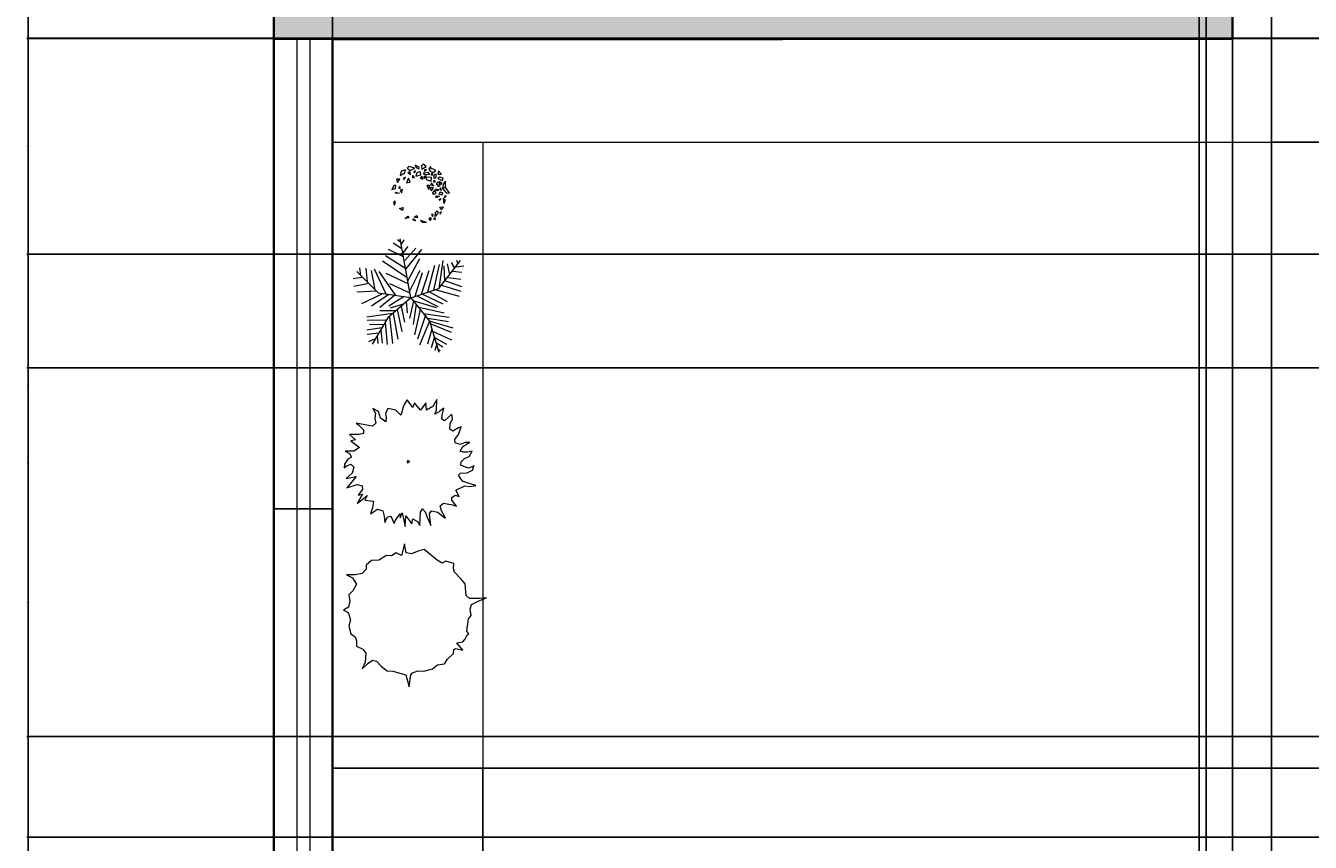
# Model space of a CAD drawing. Units: inches. Extents: x 1531 to 2263, y 2711 to 3216.
# Tile 3 of 12: x 1531 to 1728, y 2903 to 3028. Entities that reach past the tile are written whole.
import ezdxf

# ---------------------------------------------------------------- set-up
doc = ezdxf.new("R2010")
doc.units = ezdxf.units.IN
for name, color, linetype, lineweight in [('A-ANNO-DIMS', 2, 'Continuous', 18), ('A-GLAZ', 4, 'Continuous', 18), ('A-WALL', 7, 'Continuous', 35), ('L-PLNT', 94, 'Continuous', 13)]:
    doc.layers.add(name, color=color, linetype=linetype, lineweight=lineweight)
doc.layers.add('A-WALL-PATT', color=18, linetype='Continuous', lineweight=13, true_color=0x000000)
doc.styles.get("Standard").update_dxf_attribs({"font": 'arial.ttf'})
doc.dimstyles.get("Standard").update_dxf_attribs({"dimtxt": 0.18, "dimasz": 0.18, "dimexe": 0.18, "dimexo": 0.0625, "dimgap": 0.09, "dimtad": 0, "dimtih": 1, "dimtoh": 1, "dimdec": 4, "dimzin": 0, "dimdsep": 46, "dimtxsty": 'Standard', "dimcen": 0.09, "dimadec": 0, "dimazin": 0, "dimtfac": 1, "dimtdec": 4, "dimtofl": 0, "dimtmove": 0, "dimatfit": 3, "dimfxl": 1, "dimtolj": 1, "dimtzin": 0, "dimarcsym": 0})

# ---------------------------------------------------------------- blocks, each defined once
blk = doc.blocks.new('*U9')
for points in [[(-113, 281), (-131, 263), (-101, 241), (-53, 263)], [(-51, 296), (-41, 270), (-13, 257), (-5, 270), (-20, 278)], [(31, 305), (14, 287), (19, 254), (64, 281)], [(105, 283), (91, 254), (102, 235), (133, 221), (160, 239), (129, 259), (117, 254)], [(-207, 153), (-238, 151), (-229, 120)], [(-147, 248), (-191, 235), (-203, 191), (-159, 215)], [(-147, 173), (-169, 158), (-166, 144)], [(-116, 162), (-138, 114), (-99, 122)], [(-123, 219), (-97, 199), (-102, 228)], [(-73, 191), (-80, 169), (-58, 171)], [(-49, 241), (-63, 228), (-58, 217), (-46, 230)], [(1, 230), (-34, 217), (-44, 182), (7, 197)], [(19, 182), (2, 164), (28, 151)], [(35, 217), (79, 224), (97, 199), (49, 197)], [(66, 252), (47, 248), (42, 235), (59, 239)], [(43, 160), (43, 180), (67, 191), (54, 175)], [(64, 173), (64, 149), (112, 131), (117, 171)], [(117, 210), (115, 197), (126, 193), (126, 210)], [(139, 140), (138, 122), (157, 129)], [(163, 202), (139, 195), (141, 158), (165, 169)], [(189, 237), (181, 202), (217, 202)], [(199, 173), (182, 158), (229, 140), (237, 162)], [(261, 131), (234, 103), (229, 59), (266, 13), (299, 10), (263, 63), (237, 61), (261, 72)], [(-287, 46), (-250, 59), (-245, 87), (-265, 90)], [(-209, 10), (-239, 8), (-250, 21)], [(-209, 79), (-215, 59), (-200, 65)], [(-178, 46), (-202, 39), (-190, 13)], [(90, 48), (73, 90), (97, 90)], [(112, 116), (109, 94), (139, 83)], [(109, 70), (134, 68), (112, 32)], [(148, 39), (127, 10), (139, -1), (165, 10)], [(191, 43), (175, 32), (158, 54)], [(206, 127), (181, 118), (165, 105), (187, 79), (206, 90), (194, 98)], [(206, 19), (191, 4), (227, -7), (232, 13)], [(208, 65), (201, 52), (220, 39)], [(222, 120), (208, 116), (213, 98), (218, 103)], [(-255, -69), (-270, -84), (-265, -113), (-251, -89)], [(198, -20), (163, -38), (163, -18)], [(211, -45), (203, -64), (193, -53)], [(237, -130), (215, -159), (203, -132)], [(237, -45), (242, -95), (258, -64)], [(256, -16), (247, -34), (266, -23)], [(-210, -146), (-173, -135), (-178, -165)], [(-123, -225), (-113, -240), (-152, -249)], [(-65, -256), (-77, -260), (-46, -271)], [(-59, -234), (-32, -216), (-25, -242)], [(103, -240), (90, -253), (103, -269), (117, -251)], [(134, -203), (117, -207), (127, -227)], [(153, -240), (138, -253), (157, -258)], [(155, -227), (157, -183), (175, -170), (184, -187)], [(205, -205), (218, -181), (201, -192)], [(6, -269), (21, -286), (66, -289)]]:
    blk.add_lwpolyline(points, close=True)
blk = doc.blocks.new('*U8')
for p, q in [((-221.9198, 1197.3052), (-433.5526, 1338.8594)), ((-258.7244, 1362.456), (-332.3336, 1421.4348)), ((0, 0), (-266.7, 1447.8)), ((-231.1146, 1315.2628), (-166.7002, 1421.4348)), ((-129.8956, 713.6638), (-626.7704, 1032.1544)), ((-185.1152, 1008.5578), (-553.1612, 1185.4942)), ((-194.31, 1102.9442), (-65.4812, 1256.284)), ((-148.3106, 914.1968), (118.5418, 1220.9018)), ((-129.8956, 701.8528), (265.7602, 1185.4942)), ((-74.7014, 418.7444), (219.7608, 961.39)), ((-800.1, 114.3), (-1333.5, 647.7)), ((-1234.059, 536.7274), (-1252.4486, 737.2604)), ((-1105.2302, 725.4494), (-1077.6458, 395.1732)), ((-976.4268, 666.4706), (-884.4026, 194.6402)), ((-902.8176, 713.6638), (-617.5756, 100.2538)), ((-369.1382, 53.086), (-783.1836, 642.874)), ((-93.091, 489.5342), (-700.3796, 902.3858)), ((-28.6766, 171.0436), (228.9556, 678.2816)), ((256.5654, 88.4682), (449.7832, 666.4706)), ((412.9786, 147.447), (587.8068, 796.2392)), ((560.197, 182.8292), (698.2206, 819.8358)), ((685.8, 228.6), (1219.2, 914.4)), ((689.0258, 230.0224), (790.2448, 914.1968)), ((808.6344, 784.4282), (827.0494, 418.7444)), ((891.4384, 831.6214), (946.658, 572.1096)), ((983.4626, 867.0036), (1066.2666, 725.4494)), ((1029.462, 654.685), (1241.0948, 631.0884)), ((1112.2914, 760.8316), (1296.3144, 784.4282)), ((1121.4862, 925.9824), (1149.0706, 831.6214)), ((-1206.4492, 501.3198), (-1418.082, 465.9376)), ((-1031.621, 347.98), (-1399.667, 277.1902)), ((-617.5756, 607.4918), (-74.7014, 347.98)), ((-525.5514, 347.98), (-28.6766, 123.8504)), ((100.1268, 41.275), (284.1498, 619.2774)), ((845.439, 418.7444), (1241.0948, 277.1902)), ((919.0482, 501.3198), (1222.6798, 454.152)), ((-847.598, 159.2326), (-1326.0578, 135.636)), ((-718.7946, 88.4682), (-1215.644, -147.447)), ((-543.9664, 76.6572), (-967.2066, -206.4512)), ((0, 0), (-800.1, 114.3)), ((-405.9428, 53.086), (-764.794, -241.8334)), ((0, 0), (-571.5, -495.3)), ((-166.7002, 29.4894), (-543.9664, -206.4512)), ((0, 0), (685.8, 228.6)), ((0, 0), (457.2, -571.5)), ((164.5412, 41.275), (661.416, -218.2368)), ((284.1498, 88.4682), (781.0246, -147.447)), ((458.978, 147.447), (891.4384, -88.4682)), ((615.4166, 194.6402), (1185.8752, 41.275)), ((753.4148, 312.5978), (1222.6798, 159.2326)), ((-166.7002, -147.447), (-507.1618, -253.619)), ((-341.5284, -289.0012), (-221.9198, -831.6214)), ((-240.3094, -218.2368), (-157.5054, -595.7062)), ((-120.7008, -88.4682), (-93.091, -371.5766)), ((63.3222, -76.6826), (-37.8714, -513.1308)), ((44.9326, -64.897), (615.4166, -241.8334)), ((127.7366, -159.258), (54.1274, -654.685)), ((228.9556, -289.0012), (90.932, -914.1968)), ((192.151, -230.0224), (817.8292, -371.5766)), ((-442.7474, -383.3876), (-1086.8406, -477.7486)), ((-617.5756, -548.5384), (-1077.6458, -560.324)), ((-571.5, -495.3), (-952.5, -1143)), ((-387.5278, -324.4088), (-764.794, -324.4088)), ((-635.9652, -607.5172), (-580.771, -1150.1374)), ((-525.5514, -465.963), (-451.9422, -1126.5408)), ((-433.5526, -383.3876), (-323.1134, -1020.3688)), ((357.759, -430.5554), (164.5412, -1020.3688)), ((458.978, -572.1096), (210.5406, -1161.923)), ((311.7596, -383.3876), (937.4378, -477.7486)), ((412.9786, -501.3452), (919.0482, -583.9206)), ((457.2, -571.5), (685.8, -1333.5)), ((468.1982, -572.1096), (1029.462, -737.2604)), ((-718.7946, -737.2604), (-1086.8406, -796.2392)), ((-783.1836, -867.029), (-1077.6458, -902.4112)), ((-681.9646, -666.496), (-1022.4262, -654.685)), ((-829.2084, -937.7934), (-810.7934, -1126.5408)), ((-737.1842, -784.4536), (-709.5744, -1114.7298)), ((514.1976, -772.6426), (403.7838, -1138.3264)), ((486.5878, -642.8994), (983.4626, -843.4324)), ((541.8074, -831.6214), (992.6574, -1032.1544)), ((-875.2078, -1008.5832), (-1040.8412, -1079.3476)), ((578.612, -961.39), (495.7826, -1232.7128)), ((578.612, -973.1756), (873.0488, -1138.3264)), ((624.6114, -1161.923), (587.8068, -1291.6916)), ((624.6114, -1102.9442), (781.0246, -1209.1162)), ((679.8056, -1268.095), (716.6102, -1291.6916))]:
    blk.add_line(p, q)
blk = doc.blocks.new('*U10')
for points in [[(0, 1540.256), (-77.4954, 1428.4452), (-106.5784, 1341.501), (-135.636, 1217.295), (-155.0162, 1167.6126), (-280.9748, 1291.8186), (-474.7514, 1329.0804), (-532.892, 1204.8744), (-513.5118, 1105.5096), (-523.1892, 1006.1194), (-658.8506, 1093.089), (-707.2884, 1254.5568), (-842.9244, 1329.0804), (-775.1064, 1204.8744), (-794.4866, 1093.089), (-765.429, 968.8576), (-852.6272, 894.334), (-1036.701, 931.5958), (-1249.8832, 968.8576), (-1191.7426, 931.5958), (-1075.4614, 807.3898), (-1075.4614, 720.4456), (-1182.0398, 695.6044), (-1414.5768, 695.6044), (-1269.238, 558.9524), (-1385.5192, 534.1112), (-1172.3624, 372.6434), (-1307.9984, 285.6992), (-1521.1552, 285.6992), (-1414.5768, 223.5962), (-1366.139, 136.652), (-1453.3372, 86.9442), (-1540.5354, -37.2618), (-1550.2382, -124.206), (-1501.775, -86.9442), (-1385.5192, -37.2618), (-1307.9984, -111.7854), (-1346.7588, -260.8326), (-1501.775, -385.064), (-1249.8832, -335.3816), (-1482.3948, -621.0554), (-1230.503, -534.1112), (-1104.5444, -571.373), (-1094.8416, -658.3172), (-1201.42, -794.9692), (-1094.8416, -770.128), (-1230.503, -1006.1194), (-978.5858, -807.3898), (-1036.701, -919.1752), (-823.5442, -944.0164), (-852.6272, -1105.4842), (-901.065, -1254.5568), (-726.6686, -1142.746), (-600.71, -1180.0078), (-561.9496, -1316.6598), (-552.2722, -1465.707), (-484.4542, -1329.0804), (-397.2306, -1316.6598), (-319.7352, -1490.5482), (-280.9748, -1391.1834), (-174.3964, -1254.5568), (-174.3964, -1353.9216), (-125.9586, -1229.7156), (-48.4378, -1565.0718), (-29.0576, -1304.2392), (116.2812, -1502.9688), (135.6614, -1378.7628), (251.9172, -1440.8658), (310.0578, -1540.2306), (329.438, -1217.295), (377.8758, -1130.3254), (445.6938, -1204.8744), (494.157, -1341.501), (581.3552, -1540.2306), (552.2722, -1254.5568), (600.71, -1180.0078), (755.7516, -1217.295), (891.3876, -1329.0804), (939.8254, -1366.3422), (842.9498, -1180.0078), (813.8668, -1055.8018), (891.3876, -993.6988), (1114.2472, -1030.9606), (1211.1228, -1068.2224), (1094.867, -919.1752), (1094.867, -857.0722), (1182.0652, -794.9692), (1278.9408, -832.231), (1191.7426, -670.7378), (1414.6022, -571.373), (1540.5608, -583.7936), (1685.8996, -558.9524), (1521.1806, -509.27), (1375.8418, -459.5876), (1317.7012, -397.4846), (1259.5606, -310.515), (1308.0238, -260.8326), (1472.7174, -248.412), (1608.3788, -186.309), (1637.4364, -74.5236)], [(1647.1392, -74.5236), (1511.4778, -136.6266), (1433.9824, -111.7854), (1317.7012, -62.103), (1327.404, 24.8412), (1404.8994, 99.3648), (1521.1806, 149.0726), (1598.676, 285.6992), (1482.4202, 260.858), (1385.5192, 260.858), (1298.321, 285.6992), (1366.139, 397.4846), (1472.7174, 459.5876), (1540.5608, 496.8494), (1424.2796, 496.8494), (1298.321, 447.167), (1182.0652, 484.4288), (1172.3624, 571.3984), (1259.5606, 695.6044), (1327.404, 881.9134), (1259.5606, 857.0722), (1123.9246, 770.128), (1046.4038, 819.8104), (1056.1066, 956.437), (1114.2472, 1080.6684), (1094.867, 1192.4538), (1017.3462, 1117.9302), (920.4452, 1030.9606), (852.6272, 1068.2478), (862.33, 1167.6126), (901.0904, 1341.501), (794.512, 1254.5568), (678.2308, 1192.4538), (716.9912, 1291.8186), (726.6686, 1552.6766), (629.793, 1378.7628), (474.7768, 1291.8186), (455.3966, 1465.7324), (329.438, 1291.8186), (184.0992, 1465.7324), (135.6614, 1353.9216), (0, 1540.256)]]:
    blk.add_lwpolyline(points)
blk.add_lwpolyline([(9.7028, 49.6824), (0, 0), (48.4378, 12.4206), (58.1406, 37.2618)], close=True)
blk = doc.blocks.new('*U11')
blk.add_lwpolyline([(-116.2558, 1689.3032), (-193.7766, 1403.604), (-319.7352, 1465.707), (-435.991, 1391.1834), (-561.9496, 1403.604), (-746.0488, 1291.8186), (-930.1226, 1279.398), (-1056.0812, 1167.5872), (-1056.0812, 1068.2224), (-1152.9822, 956.437), (-1327.3786, 931.5958), (-1540.5354, 931.5958), (-1395.1966, 857.0722), (-1298.321, 695.579), (-1385.5192, 534.1112), (-1482.3948, 434.7464), (-1463.0146, 285.6992), (-1492.0976, 136.6266), (-1618.0562, 62.103), (-1501.775, 0), (-1443.6598, -173.8884), (-1482.3948, -335.3816), (-1433.957, -521.6906), (-1327.3786, -596.2142), (-1298.321, -695.6044), (-1298.321, -819.8104), (-1143.2794, -894.334), (-1065.784, -993.6988), (-1085.1642, -1217.295), (-1152.9822, -1378.7628), (-1027.0236, -1254.5568), (-901.065, -1167.6126), (-804.164, -1192.4538), (-687.9082, -1316.6598), (-542.5694, -1428.4452), (-406.9334, -1440.8658), (-87.1982, -1527.8354), (0, -1825.9298), (38.7604, -1527.8354), (77.5208, -1478.1276), (213.1568, -1428.4452), (358.4956, -1440.8658), (571.6524, -1378.7628), (697.611, -1279.398), (862.33, -1254.5568), (939.8508, -1142.7714), (1085.1642, -1006.1194), (1094.867, -906.7546), (1143.3048, -881.9134), (1317.7012, -919.1752), (1172.3878, -745.2868), (1317.7012, -720.4456), (1366.139, -658.3426), (1424.2796, -546.5318), (1463.04, -521.6906), (1414.6022, -459.5876), (1453.3626, -149.0472), (1521.1806, -74.5236), (1492.0976, 86.9442), (1530.858, 198.7296), (1705.2798, 285.6992), (1899.0564, 360.2228), (1724.6346, 347.8022), (1482.4202, 347.8022), (1395.222, 422.3258), (1375.8418, 707.9996), (1278.9662, 819.8104), (1114.2472, 993.6988), (1085.1642, 1080.643), (1094.867, 1204.8744), (901.0904, 1266.9774), (804.1894, 1217.295), (687.9336, 1291.8186), (368.1984, 1552.6512), (232.537, 1515.3894), (58.1406, 1440.8658), (-77.4954, 1465.707)], close=True)
blk = doc.blocks.new('WIN-72IN')
for p, q in [((0, 5.5), (72, 5.5)), ((0, 3.5), (72, 3.5))]:
    blk.add_line(p, q)
for points in [[(0, 9), (0, 0)], [(72, 0), (72, 9)]]:
    blk.add_lwpolyline(points)
blk = doc.blocks.new('*D56')
at = {"layer": 'A-ANNO-DIMS', "color": 0, "lineweight": -2, "transparency": 16777216}
for p, q in [((1568.85, 3182.67), (1531.04, 3182.67)), ((1531.22, 3182.49), (1531.22, 2972.86)), ((1531.22, 2762.85), (1531.22, 2972.49)), ((1568.85, 2762.67), (1531.04, 2762.67))]:
    blk.add_line(p, q, dxfattribs=at)
at = {"layer": 'A-ANNO-DIMS', "color": 0, "transparency": 16777216}
for points in [[(1531.19, 3182.49), (1531.25, 3182.49), (1531.22, 3182.67)], [(1531.19, 2762.85), (1531.25, 2762.85), (1531.22, 2762.67)]]:
    blk.add_solid(points, dxfattribs=at)
at = {"layer": 'Defpoints', "color": 0, "transparency": 16777216}
for p in [(1568.91, 3182.67), (1531.22, 2762.67), (1568.91, 2762.67)]:
    blk.add_point(p, dxfattribs=at)
at = {"layer": 'A-ANNO-DIMS', "color": 0, "transparency": 16777216, "insert": (1531.22, 2972.67), "char_height": 0.18, "attachment_point": 5}
blk.add_mtext('\\A1;420', dxfattribs=at)
blk = doc.blocks.new('*D57')
at = {"layer": 'A-ANNO-DIMS', "color": 0, "lineweight": -2, "transparency": 16777216}
for p, q in [((1577.91, 3029.62), (1577.91, 2711.06)), ((1711.91, 3029.69), (1711.91, 2711.06)), ((1578.09, 2711.24), (1644.63, 2711.24)), ((1711.73, 2711.24), (1645.19, 2711.24))]:
    blk.add_line(p, q, dxfattribs=at)
at = {"layer": 'A-ANNO-DIMS', "color": 0, "transparency": 16777216}
for points in [[(1578.09, 2711.27), (1578.09, 2711.21), (1577.91, 2711.24)], [(1711.73, 2711.27), (1711.73, 2711.21), (1711.91, 2711.24)]]:
    blk.add_solid(points, dxfattribs=at)
at = {"layer": 'Defpoints', "color": 0, "transparency": 16777216}
for p in [(1577.91, 3029.68), (1711.91, 3029.75), (1711.91, 2711.24)]:
    blk.add_point(p, dxfattribs=at)
at = {"layer": 'A-ANNO-DIMS', "color": 0, "transparency": 16777216, "insert": (1644.91, 2711.24), "char_height": 0.18, "attachment_point": 5}
blk.add_mtext('\\A1;134', dxfattribs=at)
blk = doc.blocks.new('*D58')
at = {"layer": 'A-ANNO-DIMS', "color": 0, "lineweight": -2, "transparency": 16777216}
for p, q in [((1715.91, 3097.69), (1715.91, 2711.06)), ((1775.91, 3097.72), (1775.91, 2711.06)), ((1716.09, 2711.24), (1745.69, 2711.24)), ((1775.73, 2711.24), (1746.13, 2711.24))]:
    blk.add_line(p, q, dxfattribs=at)
at = {"layer": 'A-ANNO-DIMS', "color": 0, "transparency": 16777216}
for points in [[(1716.09, 2711.27), (1716.09, 2711.21), (1715.91, 2711.24)], [(1775.73, 2711.27), (1775.73, 2711.21), (1775.91, 2711.24)]]:
    blk.add_solid(points, dxfattribs=at)
at = {"layer": 'Defpoints', "color": 0, "transparency": 16777216}
for p in [(1715.91, 3097.75), (1775.91, 3097.78), (1775.91, 2711.24)]:
    blk.add_point(p, dxfattribs=at)
at = {"layer": 'A-ANNO-DIMS', "color": 0, "transparency": 16777216, "insert": (1745.91, 2711.24), "char_height": 0.18, "attachment_point": 5}
blk.add_mtext('\\A1;60', dxfattribs=at)
blk = doc.blocks.new('*D64')
at = {"layer": 'A-ANNO-DIMS', "color": 0, "lineweight": -2, "transparency": 16777216}
for p, q in [((1779.85, 3025.79), (1531.04, 3025.79)), ((1531.22, 3025.61), (1531.22, 2960.97)), ((1531.22, 2895.96), (1531.22, 2960.6)), ((1775.85, 2895.78), (1531.04, 2895.78))]:
    blk.add_line(p, q, dxfattribs=at)
at = {"layer": 'A-ANNO-DIMS', "color": 0, "transparency": 16777216}
for points in [[(1531.19, 3025.61), (1531.25, 3025.61), (1531.22, 3025.79)], [(1531.19, 2895.96), (1531.25, 2895.96), (1531.22, 2895.78)]]:
    blk.add_solid(points, dxfattribs=at)
at = {"layer": 'Defpoints', "color": 0, "transparency": 16777216}
for p in [(1779.91, 3025.79), (1531.22, 2895.78), (1775.91, 2895.78)]:
    blk.add_point(p, dxfattribs=at)
at = {"layer": 'A-ANNO-DIMS', "color": 0, "transparency": 16777216, "insert": (1531.22, 2960.78), "char_height": 0.18, "attachment_point": 5}
blk.add_mtext('\\A1;130', dxfattribs=at)
blk = doc.blocks.new('*D66')
at = {"layer": 'A-ANNO-DIMS', "color": 0, "lineweight": -2, "transparency": 16777216}
for p, q in [((1577.91, 2895.74), (1577.91, 3216.47)), ((1578.09, 3216.29), (1676.63, 3216.29)), ((1775.73, 3216.29), (1677.19, 3216.29)), ((1775.91, 2895.85), (1775.91, 3216.47))]:
    blk.add_line(p, q, dxfattribs=at)
at = {"layer": 'A-ANNO-DIMS', "color": 0, "transparency": 16777216}
for points in [[(1578.09, 3216.32), (1578.09, 3216.26), (1577.91, 3216.29)], [(1775.73, 3216.32), (1775.73, 3216.26), (1775.91, 3216.29)]]:
    blk.add_solid(points, dxfattribs=at)
at = {"layer": 'Defpoints', "color": 0, "transparency": 16777216}
for p in [(1775.91, 3216.29), (1577.91, 2895.68), (1775.91, 2895.78)]:
    blk.add_point(p, dxfattribs=at)
at = {"layer": 'A-ANNO-DIMS', "color": 0, "transparency": 16777216, "insert": (1676.91, 3216.29), "char_height": 0.18, "attachment_point": 5}
blk.add_mtext('\\A1;198', dxfattribs=at)
blk = doc.blocks.new('*D77')
at = {"layer": 'A-ANNO-DIMS', "color": 0, "lineweight": -2, "transparency": 16777216}
for p, q in [((2094.81, 2975.33), (1531.04, 2975.33)), ((1531.22, 2975.15), (1531.22, 2939.52)), ((1531.22, 2903.53), (1531.22, 2939.16)), ((2094.81, 2903.35), (1531.04, 2903.35))]:
    blk.add_line(p, q, dxfattribs=at)
at = {"layer": 'A-ANNO-DIMS', "color": 0, "transparency": 16777216}
for points in [[(1531.19, 2975.15), (1531.25, 2975.15), (1531.22, 2975.33)], [(1531.19, 2903.53), (1531.25, 2903.53), (1531.22, 2903.35)]]:
    blk.add_solid(points, dxfattribs=at)
at = {"layer": 'Defpoints', "color": 0, "transparency": 16777216}
for p in [(2094.87, 2975.33), (1531.22, 2903.35), (2094.87, 2903.35)]:
    blk.add_point(p, dxfattribs=at)
at = {"layer": 'A-ANNO-DIMS', "color": 0, "transparency": 16777216, "insert": (1531.22, 2939.34), "char_height": 0.18, "attachment_point": 5}
blk.add_mtext('\\A1;71.98', dxfattribs=at)
blk = doc.blocks.new('*D87')
at = {"layer": 'A-ANNO-DIMS', "color": 0, "lineweight": -2, "transparency": 16777216}
for p, q in [((1721.91, 3101.69), (1721.91, 2711.06)), ((1745.91, 3101.7), (1745.91, 2711.06)), ((1722.09, 2711.24), (1733.69, 2711.24)), ((1745.73, 2711.24), (1734.13, 2711.24))]:
    blk.add_line(p, q, dxfattribs=at)
at = {"layer": 'A-ANNO-DIMS', "color": 0, "transparency": 16777216}
for points in [[(1722.09, 2711.27), (1722.09, 2711.21), (1721.91, 2711.24)], [(1745.73, 2711.27), (1745.73, 2711.21), (1745.91, 2711.24)]]:
    blk.add_solid(points, dxfattribs=at)
at = {"layer": 'Defpoints', "color": 0, "transparency": 16777216}
for p in [(1721.91, 3101.75), (1745.91, 3101.77), (1745.91, 2711.24)]:
    blk.add_point(p, dxfattribs=at)
at = {"layer": 'A-ANNO-DIMS', "color": 0, "transparency": 16777216, "insert": (1733.91, 2711.24), "char_height": 0.18, "attachment_point": 5}
blk.add_mtext('\\A1;24', dxfattribs=at)
blk = doc.blocks.new('*D101')
at = {"layer": 'A-ANNO-DIMS', "color": 0, "lineweight": -2, "transparency": 16777216}
for p, q in [((2228.85, 2918.81), (1531.04, 2918.81)), ((1531.22, 2918.63), (1531.22, 2897.08)), ((1531.22, 2875.18), (1531.22, 2896.72)), ((2228.85, 2875), (1531.04, 2875))]:
    blk.add_line(p, q, dxfattribs=at)
at = {"layer": 'A-ANNO-DIMS', "color": 0, "transparency": 16777216}
for points in [[(1531.19, 2918.63), (1531.25, 2918.63), (1531.22, 2918.81)], [(1531.19, 2875.18), (1531.25, 2875.18), (1531.22, 2875)]]:
    blk.add_solid(points, dxfattribs=at)
at = {"layer": 'Defpoints', "color": 0, "transparency": 16777216}
for p in [(2228.91, 2918.81), (1531.22, 2875), (2228.91, 2875)]:
    blk.add_point(p, dxfattribs=at)
at = {"layer": 'A-ANNO-DIMS', "color": 0, "transparency": 16777216, "insert": (1531.22, 2896.9), "char_height": 0.18, "attachment_point": 5}
blk.add_mtext('\\A1;43.81', dxfattribs=at)
blk = doc.blocks.new('*D111')
at = {"layer": 'A-ANNO-DIMS', "color": 0, "lineweight": -2, "transparency": 16777216}
for p, q in [((1577.91, 3010), (1577.91, 3216.47)), ((1578.09, 3216.29), (1649.63, 3216.29)), ((1721.73, 3216.29), (1650.19, 3216.29)), ((1721.91, 3010), (1721.91, 3216.47))]:
    blk.add_line(p, q, dxfattribs=at)
at = {"layer": 'A-ANNO-DIMS', "color": 0, "transparency": 16777216}
for points in [[(1578.09, 3216.32), (1578.09, 3216.26), (1577.91, 3216.29)], [(1721.73, 3216.32), (1721.73, 3216.26), (1721.91, 3216.29)]]:
    blk.add_solid(points, dxfattribs=at)
at = {"layer": 'Defpoints', "color": 0, "transparency": 16777216}
for p in [(1721.91, 3216.29), (1577.91, 3009.94), (1721.91, 3009.94)]:
    blk.add_point(p, dxfattribs=at)
at = {"layer": 'A-ANNO-DIMS', "color": 0, "transparency": 16777216, "insert": (1649.91, 3216.29), "char_height": 0.18, "attachment_point": 5}
blk.add_mtext('\\A1;144', dxfattribs=at)
blk = doc.blocks.new('*D112')
at = {"layer": 'A-ANNO-DIMS', "color": 0, "lineweight": -2, "transparency": 16777216}
for p, q in [((1721.97, 3009.94), (2262.37, 3009.94)), ((2262.19, 3009.76), (2262.19, 2962.12)), ((2262.19, 2914.12), (2262.19, 2961.76)), ((1721.97, 2913.94), (2262.37, 2913.94))]:
    blk.add_line(p, q, dxfattribs=at)
at = {"layer": 'A-ANNO-DIMS', "color": 0, "transparency": 16777216}
for points in [[(2262.16, 3009.76), (2262.22, 3009.76), (2262.19, 3009.94)], [(2262.16, 2914.12), (2262.22, 2914.12), (2262.19, 2913.94)]]:
    blk.add_solid(points, dxfattribs=at)
at = {"layer": 'Defpoints', "color": 0, "transparency": 16777216}
for p in [(1721.91, 3009.94), (1721.91, 2913.94), (2262.19, 2913.94)]:
    blk.add_point(p, dxfattribs=at)
at = {"layer": 'A-ANNO-DIMS', "color": 0, "transparency": 16777216, "insert": (2262.19, 2961.94), "char_height": 0.18, "attachment_point": 5}
blk.add_mtext('\\A1;96', dxfattribs=at)
blk = doc.blocks.new('*D113')
at = {"layer": 'A-ANNO-DIMS', "color": 0, "lineweight": -2, "transparency": 16777216}
for p, q in [((1577.91, 2913.88), (1577.91, 2711.06)), ((1600.94, 2913.88), (1600.94, 2711.06)), ((1578.09, 2711.24), (1588.96, 2711.24)), ((1600.76, 2711.24), (1589.89, 2711.24))]:
    blk.add_line(p, q, dxfattribs=at)
at = {"layer": 'A-ANNO-DIMS', "color": 0, "transparency": 16777216}
for points in [[(1578.09, 2711.27), (1578.09, 2711.21), (1577.91, 2711.24)], [(1600.76, 2711.27), (1600.76, 2711.21), (1600.94, 2711.24)]]:
    blk.add_solid(points, dxfattribs=at)
at = {"layer": 'Defpoints', "color": 0, "transparency": 16777216}
for p in [(1577.91, 2913.94), (1600.94, 2913.94), (1600.94, 2711.24)]:
    blk.add_point(p, dxfattribs=at)
at = {"layer": 'A-ANNO-DIMS', "color": 0, "transparency": 16777216, "insert": (1589.43, 2711.24), "char_height": 0.18, "attachment_point": 5}
blk.add_mtext('\\A1;23.034', dxfattribs=at)
blk = doc.blocks.new('*D114')
at = {"layer": 'A-ANNO-DIMS', "color": 0, "lineweight": -2, "transparency": 16777216}
for p, q in [((1577.97, 2913.94), (2262.37, 2913.94)), ((2262.19, 2913.76), (2262.19, 2904.99)), ((2262.19, 2895.86), (2262.19, 2904.63)), ((1577.97, 2895.68), (2262.37, 2895.68))]:
    blk.add_line(p, q, dxfattribs=at)
at = {"layer": 'A-ANNO-DIMS', "color": 0, "transparency": 16777216}
for points in [[(2262.16, 2913.76), (2262.22, 2913.76), (2262.19, 2913.94)], [(2262.16, 2895.86), (2262.22, 2895.86), (2262.19, 2895.68)]]:
    blk.add_solid(points, dxfattribs=at)
at = {"layer": 'Defpoints', "color": 0, "transparency": 16777216}
for p in [(1577.91, 2913.94), (1577.91, 2895.68), (2262.19, 2895.68)]:
    blk.add_point(p, dxfattribs=at)
at = {"layer": 'A-ANNO-DIMS', "color": 0, "transparency": 16777216, "insert": (2262.19, 2904.81), "char_height": 0.18, "attachment_point": 5}
blk.add_mtext('\\A1;18.26', dxfattribs=at)
blk = doc.blocks.new('*D122')
at = {"layer": 'A-ANNO-DIMS', "color": 0, "lineweight": -2, "transparency": 16777216}
for p, q in [((1955.85, 3025.88), (1531.04, 3025.88)), ((1531.22, 3025.7), (1531.22, 3009.49)), ((1531.22, 2992.91), (1531.22, 3009.12)), ((1968.31, 2992.73), (1531.04, 2992.73))]:
    blk.add_line(p, q, dxfattribs=at)
at = {"layer": 'A-ANNO-DIMS', "color": 0, "transparency": 16777216}
for points in [[(1531.19, 3025.7), (1531.25, 3025.7), (1531.22, 3025.88)], [(1531.19, 2992.91), (1531.25, 2992.91), (1531.22, 2992.73)]]:
    blk.add_solid(points, dxfattribs=at)
at = {"layer": 'Defpoints', "color": 0, "transparency": 16777216}
for p in [(1531.22, 3025.88), (1955.91, 3025.88), (1968.37, 2992.73)]:
    blk.add_point(p, dxfattribs=at)
at = {"layer": 'A-ANNO-DIMS', "color": 0, "transparency": 16777216, "insert": (1531.22, 3009.3), "char_height": 0.18, "attachment_point": 5}
blk.add_mtext('\\A1;33.146', dxfattribs=at)
blk = doc.blocks.new('*D128')
at = {"layer": 'A-ANNO-DIMS', "color": 0, "lineweight": -2, "transparency": 16777216}
for p, q in [((1710.84, 2841.9), (1710.84, 3216.47)), ((1711.02, 3216.29), (1721.3, 3216.29)), ((1732.52, 3216.29), (1722.23, 3216.29)), ((1732.7, 2841.9), (1732.7, 3216.47))]:
    blk.add_line(p, q, dxfattribs=at)
at = {"layer": 'A-ANNO-DIMS', "color": 0, "transparency": 16777216}
for points in [[(1711.02, 3216.32), (1711.02, 3216.26), (1710.84, 3216.29)], [(1732.52, 3216.32), (1732.52, 3216.26), (1732.7, 3216.29)]]:
    blk.add_solid(points, dxfattribs=at)
at = {"layer": 'Defpoints', "color": 0, "transparency": 16777216}
for p in [(1732.7, 3216.29), (1710.84, 2841.84), (1732.7, 2841.84)]:
    blk.add_point(p, dxfattribs=at)
at = {"layer": 'A-ANNO-DIMS', "color": 0, "transparency": 16777216, "insert": (1721.77, 3216.29), "char_height": 0.18, "attachment_point": 5}
blk.add_mtext('\\A1;21.866', dxfattribs=at)

msp = doc.modelspace()

# ---------------------------------------------------------------- hatches: boundary and pattern name
at = {"layer": 'A-WALL-PATT'}
h = msp.add_hatch(color=256, dxfattribs=at)
h.dxf.hatch_style = 1
h.paths.add_polyline_path([(1715.9101, 3035.7517), (1711.9101, 3035.7496), (1711.9101, 3029.7496), (1673.9111, 3029.7297), (1673.9111, 3029.6795), (1577.9111, 3029.6795), (1577.9111, 3050.6795), (1577.9111, 3061.3695), (1568.9111, 3061.3695), (1568.9111, 3025.6795), (1577.9111, 3025.6795), (1715.9101, 3025.7517)])

# ---------------------------------------------------------------- linework, layer by layer
at = {"layer": 'A-GLAZ'}
for p, q in [((1572.4111, 2953.6795), (1572.4111, 2895.6795)), ((1574.4111, 2953.6795), (1574.4111, 2895.6795))]:
    msp.add_line(p, q, dxfattribs=at)
msp.add_lwpolyline([(1577.9111, 2953.6795), (1568.9111, 2953.6795)], dxfattribs=at)
at = {"layer": 'A-WALL'}
for p, q in [((1715.9101, 3035.7517), (1715.9101, 3025.7517)), ((1577.9111, 3025.6795), (1715.9101, 3025.7517)), ((1577.9111, 2895.6796), (1577.9111, 3025.6795))]:
    msp.add_line(p, q, dxfattribs=at)
msp.add_lwpolyline([(1933.9101, 2762.8657), (1568.9111, 2762.6748), (1568.9111, 3182.6749), (2228.9101, 3183.02), (2228.9101, 2798.8631)], dxfattribs=at)
at = {"layer": 'L-PLNT'}
msp.add_line((1600.9446, 3009.9378), (1600.9446, 2913.9378), dxfattribs=at)
msp.add_lwpolyline([(1577.9111, 3009.9378), (1721.9111, 3009.9378), (1721.9111, 2913.9378), (1577.9111, 2913.9378)], close=True, dxfattribs=at)

# ---------------------------------------------------------------- block references
at = {"layer": 'A-GLAZ', "rotation": 270.0000000000002}
msp.add_blockref('WIN-72IN', (1568.911, 3025.6794), dxfattribs=at)
at = {"layer": 'L-PLNT'}
for name, p, xscale, yscale, zscale in [('*U9', (1591.3245, 3001.952), 0.0150576283247315, 0.0150576283247315, 0.0150576283247315), ('*U8', (1589.9341, 2986.0635), 0.0062442477113808, 0.0062442477113808, 0.0062442477113808), ('*U10', (1589.3512, 2960.774), 0.0062442477113808, 0.0062442477113808, 0.0062442477113808), ('*U11', (1589.6727, 2937.7851), 0.0062442477113808, 0.0062442477113808, 0.0062442477113808)]:
    msp.add_blockref(name, p, dxfattribs=dict(at, xscale=xscale, yscale=yscale, zscale=zscale))

# ---------------------------------------------------------------- dimensions: what is measured, and where the dimension line sits
at = {"layer": 'A-ANNO-DIMS'}
for base, p1, p2, override, picture, middle in [((1775.9101, 3216.295), (1577.9111, 2895.6796), (1775.9101, 2895.7831), {"dimdec": 0, "dimlfac": 1, "dimrnd": 0, "dimzin": 0, "dimdsep": 46, "dimlunit": 2}, '*D66', (1676.9106, 3216.295)), ((1721.9111, 3216.295), (1577.9111, 3009.9378), (1721.9111, 3009.9378), {"dimdec": 0, "dimlfac": 1, "dimrnd": 0, "dimzin": 0, "dimdsep": 46, "dimlunit": 2}, '*D111', (1649.9111, 3216.295)), ((1732.7021, 3216.295), (1710.8363, 2841.8359), (1732.7021, 2841.8359), {"dimdec": 3, "dimlfac": 1, "dimrnd": 0, "dimzin": 0, "dimdsep": 46, "dimlunit": 2}, '*D128', (1721.7692, 3216.295)), ((1745.9101, 2711.2407), (1721.9101, 3101.7549), (1745.9101, 3101.7674), {"dimdec": 0, "dimlfac": 1, "dimrnd": 0, "dimzin": 0, "dimdsep": 46, "dimlunit": 2}, '*D87', (1733.9101, 2711.2407)), ((1775.9101, 2711.2407), (1715.9101, 3097.7517), (1775.9101, 3097.7831), {"dimdec": 0, "dimlfac": 1, "dimrnd": 0, "dimzin": 0, "dimdsep": 46, "dimlunit": 2}, '*D58', (1745.9101, 2711.2407)), ((1711.9101, 2711.2407), (1577.9111, 3029.6795), (1711.9101, 3029.7496), {"dimdec": 0, "dimlfac": 1, "dimrnd": 0, "dimzin": 0, "dimdsep": 46, "dimlunit": 2}, '*D57', (1644.9106, 2711.2407)), ((1600.9446, 2711.24067), (1577.91107, 2913.93777), (1600.9446, 2913.93777), {"dimdec": 3, "dimlfac": 1, "dimrnd": 0, "dimzin": 0, "dimdsep": 46, "dimlunit": 2}, '*D113', (1589.42783, 2711.24067))]:
    dim = msp.add_linear_dim(base=base, p1=p1, p2=p2, dimstyle='Standard', override=override, dxfattribs=at)
    dim.commit()
    dim.dimension.update_dxf_attribs({"geometry": picture, "text_midpoint": middle})
for base, p1, p2, override, picture, middle in [((1531.2212, 2762.6748), (1568.9111, 3182.6749), (1568.9111, 2762.6748), {"dimdec": 0, "dimlfac": 1, "dimrnd": 0, "dimzin": 0, "dimdsep": 46, "dimlunit": 2}, '*D56', (1531.2212, 2972.6748)), ((1531.2212, 3025.8772), (1968.3722, 2992.7314), (1955.9101, 3025.8772), {"dimdec": 3, "dimlfac": 1, "dimrnd": 0, "dimzin": 0, "dimdsep": 46, "dimlunit": 2}, '*D122', (1531.2212, 3009.3043)), ((1531.2212, 2895.7831), (1779.9101, 3025.7852), (1775.9101, 2895.7831), {"dimdec": 0, "dimlfac": 1, "dimrnd": 0, "dimzin": 0, "dimdsep": 46, "dimlunit": 2}, '*D64', (1531.2212, 2960.7841)), ((2262.1851, 2913.9378), (1721.9111, 3009.9378), (1721.9111, 2913.9378), {"dimdec": 0, "dimlfac": 1, "dimrnd": 0, "dimzin": 0, "dimdsep": 46, "dimlunit": 2}, '*D112', (2262.1851, 2961.9378)), ((1531.2212, 2903.3482), (2094.8725, 2975.3315), (2094.8725, 2903.3482), {"dimdec": 2, "dimlfac": 1, "dimrnd": 0, "dimzin": 0, "dimdsep": 46, "dimlunit": 2}, '*D77', (1531.2212, 2939.3398)), ((1531.2212, 2874.9957), (2228.9101, 2918.8056), (2228.9101, 2874.9957), {"dimdec": 2, "dimlfac": 1, "dimrnd": 0, "dimzin": 0, "dimdsep": 46, "dimlunit": 2}, '*D101', (1531.2212, 2896.9007)), ((2262.1851, 2895.6796), (1577.9111, 2913.9378), (1577.9111, 2895.6796), {"dimdec": 2, "dimlfac": 1, "dimrnd": 0, "dimzin": 0, "dimdsep": 46, "dimlunit": 2}, '*D114', (2262.1851, 2904.8087))]:
    dim = msp.add_linear_dim(base=base, p1=p1, p2=p2, angle=90, dimstyle='Standard', override=override, dxfattribs=at)
    dim.commit()
    dim.dimension.update_dxf_attribs({"geometry": picture, "text_midpoint": middle})

doc.saveas('drawing.dxf')
